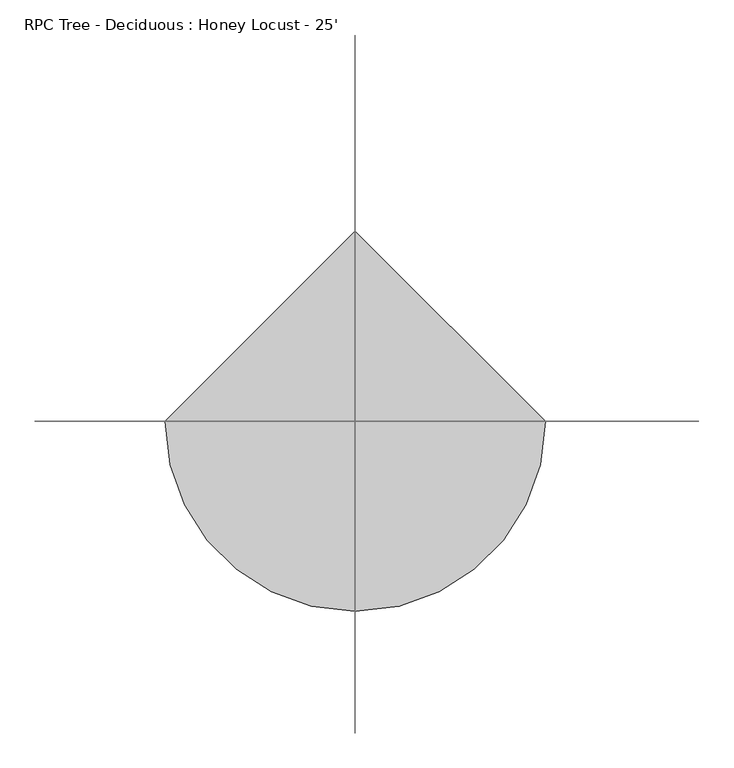
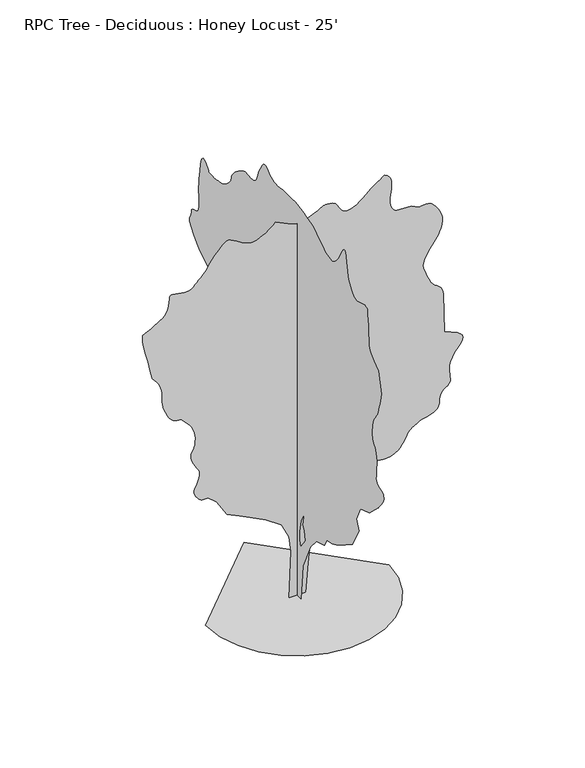
"""IFC4 building model written with IfcOpenShell, lengths in millimetres: geographic element geometry, RPC Tree - Deciduous : Honey Locust - 25'."""

from ifc_helpers import new_model, si_unit, origin, place, context, project, spatial, triangles, source, transform, mapped, element, save


def rpc_tree_deciduous_honey_locust_25_cc46a1f1(model_context):
    return source(origin(), model_context, "Body", "Tessellation", [
        triangles([(0.0017564, 138.2462219, 0.0), (0.0017564, -127.0105432, 0.0), (0.0017564, -184.6753374, 668.9082985), (0.0017564, -426.8668951, 1176.3566122), (0.0017564, -611.3926231, 1395.4822632), (0.0017564, -865.1155083, 1476.2135273), (0.0017564, -934.3152088, 1614.6078415), (0.0017564, -1118.8409369, 1660.7391827), (0.0017564, -1168.1321142, 1679.0297813), (0.0017564, -1234.9772346, 1712.4509972), (0.0017564, -1316.4476978, 1758.4833618), (0.0017564, -1409.6173016, 1814.6021748), (0.0017564, -1511.5651485, 1878.2849155), (0.0017564, -1619.3626385, 1947.0122612), (0.0017564, -1730.0862579, 2018.2590752), (0.0017564, -1937.6776566, 2398.8447109), (0.0017564, -1856.9463924, 2583.3806854), (0.0017564, -1983.8091431, 2848.632518), (0.0017564, -2272.1318058, 2952.4168808), (0.0017564, -2537.389016, 3206.1371498), (0.0017564, -2543.9089668, 3214.0110878), (0.0017564, -2561.3334846, 3235.1946785), (0.0017564, -2586.4031754, 3266.0558762), (0.0017564, -2615.9435234, 3302.9873428), (0.0017564, -2646.6774033, 3342.3317436), (0.0017564, -2675.3794304, 3380.4573235), (0.0017564, -2698.8489281, 3413.7311646), (0.0017564, -2714.4444878, 3444.5414932), (0.0017564, -2721.9882133, 3476.5453537), (0.0017564, -2721.8358971, 3508.1684235), (0.0017564, -2714.4444878, 3537.73377), (0.0017564, -2700.1950668, 3563.6926506), (0.0017564, -2679.4940048, 3584.4190018), (0.0017564, -2652.7226738, 3598.2620522), (0.0017564, -2621.3536583, 3608.345739), (0.0017564, -2588.1556847, 3619.6488281), (0.0017564, -2555.5675575, 3633.3648514), (0.0017564, -2526.024884, 3650.7129204), (0.0017564, -2501.9153091, 3672.9124374), (0.0017564, -2485.67444, 3701.157225), (0.0017564, -2479.7233498, 3736.6663948), (0.0017564, -2481.5749809, 3780.2273987), (0.0017564, -2486.0453476, 3831.0780739), (0.0017564, -2491.5266991, 3887.9740196), (0.0017564, -2496.4008202, 3949.6961243), (0.0017564, -2499.0579254, 4015.0755638), (0.0017564, -2497.8818344, 4082.8426483), (0.0017564, -2491.2575294, 4151.8544243), (0.0017564, -2477.5720276, 4213.7541344), (0.0017564, -2458.0368828, 4262.9284584), (0.0017564, -2435.2733013, 4302.24757), (0.0017564, -2411.9053963, 4334.4801956), (0.0017564, -2390.5542286, 4362.4965088), (0.0017564, -2373.8434753, 4389.0902344), (0.0017564, -2364.3947788, 4417.1062569), (0.0017564, -2359.5864967, 4450.1263344), (0.0017564, -2355.5860142, 4489.1913918), (0.0017564, -2353.1983692, 4533.3113731), (0.0017564, -2353.2315067, 4581.4694801), (0.0017564, -2356.4927902, 4632.6250786), (0.0017564, -2363.7901646, 4685.8128204), (0.0017564, -2375.9288132, 4740.016198), (0.0017564, -2392.0679443, 4787.9461212), (0.0017564, -2410.4271435, 4825.3601166), (0.0017564, -2430.3991802, 4855.916391), (0.0017564, -2451.3794403, 4883.2722794), (0.0017564, -2472.7636002, 4911.0089584), (0.0017564, -2493.9471909, 4942.7843445), (0.0017564, -2514.3232727, 4982.2051941), (0.0017564, -2534.0944496, 5031.4045166), (0.0017564, -2553.8659172, 5089.0626251), (0.0017564, -2573.6269203, 5153.8075104), (0.0017564, -2593.4135033, 5224.1654251), (0.0017564, -2613.1747971, 5298.7905212), (0.0017564, -2632.9360909, 5376.2096329), (0.0017564, -2652.7226738, 5455.0763306), (0.0017564, -2548.9127312, 5835.6443802), (0.0017564, -2410.52612, 5939.4537415), (0.0017564, -2376.165136, 5966.8602081), (0.0017564, -2343.2136589, 5995.5625259), (0.0017564, -2313.0867188, 6026.9059616), (0.0017564, -2287.1965839, 6062.1863663), (0.0017564, -2266.9553776, 6102.6995911), (0.0017564, -2253.772752, 6149.7659042), (0.0017564, -2249.0662079, 6204.705574), (0.0017564, -2247.7225399, 6269.3992996), (0.0017564, -2243.9556187, 6343.7709229), (0.0017564, -2238.1721054, 6426.2187973), (0.0017564, -2230.7756092, 6515.1186035), (0.0017564, -2222.1675591, 6608.8704391), (0.0017564, -2212.7518547, 6705.8220795), (0.0017564, -2202.9347214, 6804.4247818), (0.0017564, -2185.5179066, 6814.1270966), (0.0017564, -2167.3950302, 6822.8393555), (0.0017564, -2147.8598854, 6829.5453415), (0.0017564, -2126.2064106, 6833.2026764), (0.0017564, -2101.7285442, 6832.8218857), (0.0017564, -2073.7199341, 6827.4117508), (0.0017564, -2041.4746639, 6815.9560547), (0.0017564, -2006.8748863, 6801.3255524), (0.0017564, -1972.2775795, 6787.914743), (0.0017564, -1937.6776566, 6776.9165771), (0.0017564, -1903.077879, 6769.5501663), (0.0017564, -1868.4805721, 6767.0357849), (0.0017564, -1833.8806492, 6770.5663834), (0.0017564, -1799.2833424, 6781.3616547), (0.0017564, -1765.6919334, 6801.5546082), (0.0017564, -1733.9191635, 6831.4504578), (0.0017564, -1703.6576385, 6869.42314), (0.0017564, -1674.6050514, 6913.8221741), (0.0017564, -1646.4618565, 6963.0982361), (0.0017564, -1618.9257465, 7015.5746841), (0.0017564, -1591.689473, 7069.6766144), (0.0017564, -1522.4922432, 7484.8646439), (0.0017564, -1510.0182953, 7494.262326), (0.0017564, -1496.8382858, 7500.8665741), (0.0017564, -1482.2460079, 7501.8060516), (0.0017564, -1465.5354, 7494.262326), (0.0017564, -1446.0002552, 7475.4413818), (0.0017564, -1422.9345119, 7442.4974625), (0.0017564, -1395.6321087, 7392.5865555), (0.0017564, -1366.480545, 7335.9952423), (0.0017564, -1337.5296959, 7284.4588531), (0.0017564, -1307.5703327, 7237.3669601), (0.0017564, -1275.393663, 7194.085881), (0.0017564, -1239.7855167, 7154.0296051), (0.0017564, -1199.5366653, 7116.6156097), (0.0017564, -1153.4407871, 7081.2078873), (0.0017564, -1100.9873028, 7057.7133911), (0.0017564, -1043.0880753, 7054.1827927), (0.0017564, -980.6472645, 7067.2889694), (0.0017564, -914.5768787, 7093.7047989), (0.0017564, -845.7836214, 7130.1287384), (0.0017564, -775.1741959, 7173.2069229), (0.0017564, -703.6555235, 7219.6128113), (0.0017564, -659.2741482, 7251.5405136), (0.0017564, -615.4946983, 7282.3758408), (0.0017564, -572.9269114, 7311.0014191), (0.0017564, -532.1751838, 7336.2748764), (0.0017564, -493.8440932, 7357.1282547), (0.0017564, -458.5406522, 7372.4186005), (0.0017564, -426.8668951, 7381.0547012), (0.0017564, -379.7931333, 7391.6464966), (0.0017564, -304.4771091, 7410.7220764), (0.0017564, -210.8004869, 7434.013678), (0.0017564, -108.6519436, 7457.3308594), (0.0017564, -7.915369, 7476.3808594), (0.0017564, 81.5235032, 7486.9726547), (0.0017564, 149.779584, 7484.8646439), (0.0017564, 204.0816928, 7478.1336594), (0.0017564, 257.9799291, 7476.2541229), (0.0017564, 311.0709472, 7476.9907059), (0.0017564, 362.9529548, 7478.1336594), (0.0017564, 413.2194723, 7477.4732346), (0.0017564, 461.4692888, 7472.7485229), (0.0017564, 507.2984682, 7461.8015167), (0.0017564, 555.4821914, 7451.6666702), (0.0017564, 608.9110522, 7450.0156082), (0.0017564, 664.3541433, 7455.4513229), (0.0017564, 718.5906584, 7466.5000671), (0.0017564, 768.3873281, 7481.7909943), (0.0017564, 810.5182594, 7499.9265152), (0.0017564, 841.7526175, 7519.4590439), (0.0017564, 869.6950979, 7543.2081757), (0.0017564, 902.8827524, 7570.9704346), (0.0017564, 939.4967966, 7596.9293152), (0.0017564, 977.728838, 7615.2171524), (0.0017564, 1015.7551506, 7619.9924423), (0.0017564, 1051.7671967, 7605.3875198), (0.0017564, 1083.943939, 7565.5858795), (0.0017564, 1111.584185, 7516.9952408), (0.0017564, 1135.5896965, 7477.701709), (0.0017564, 1156.5725727, 7444.2496811), (0.0017564, 1175.132341, 7413.2114594), (0.0017564, 1191.8760138, 7381.1564392), (0.0017564, 1207.410676, 7344.6819214), (0.0017564, 1222.3407967, 7300.3334656), (0.0017564, 1236.6967518, 7254.9693741), (0.0017564, 1251.0554684, 7217.07285), (0.0017564, 1266.8236919, 7185.6526749), (0.0017564, 1285.4164524, 7159.6432159), (0.0017564, 1308.248489, 7138.103833), (0.0017564, 1336.7269833, 7119.9683121), (0.0017564, 1372.2666744, 7104.2710144), (0.0017564, 1413.6914715, 7095.1529663), (0.0017564, 1457.9408054, 7094.9239105), (0.0017564, 1503.6022625, 7099.7247803), (0.0017564, 1549.2612488, 7105.7447617), (0.0017564, 1593.5105827, 7109.1480423), (0.0017564, 1634.9353798, 7106.0999725), (0.0017564, 1672.1235168, 7092.7397415), (0.0017564, 1714.3205051, 7068.3051865), (0.0017564, 1768.2192501, 7035.5897415), (0.0017564, 1828.5747231, 6996.1944717), (0.0017564, 1890.1391338, 6951.7954376), (0.0017564, 1947.6700699, 6903.9419632), (0.0017564, 1995.9198864, 6854.2845291), (0.0017564, 2029.6434093, 6804.4247818), (0.0017564, 2047.5985634, 6762.5657089), (0.0017564, 2056.0720287, 6732.1873306), (0.0017564, 2061.1140175, 6707.879512), (0.0017564, 2068.7821541, 6684.1809586), (0.0017564, 2085.1219997, 6655.6315384), (0.0017564, 2116.1913242, 6616.7949554), (0.0017564, 2168.0377235, 6562.2360764), (0.0017564, 2230.1762272, 6507.9306702), (0.0017564, 2288.0754547, 6470.9736237), (0.0017564, 2341.7380222, 6447.5297058), (0.0017564, 2391.1637844, 6433.7881027), (0.0017564, 2436.3553574, 6425.8885849), (0.0017564, 2477.3077995, 6419.9959213), (0.0017564, 2514.0259071, 6412.2998795), (0.0017564, 2553.510125, 6405.0352066), (0.0017564, 2599.6366699, 6402.2161926), (0.0017564, 2647.7694878, 6402.6225632), (0.0017564, 2693.3117661, 6405.0352066), (0.0017564, 2731.5640823, 6408.2611725), (0.0017564, 2757.9293335, 6411.0807678), (0.0017564, 2767.7589661, 6412.2998795), (0.0017564, 2779.3922676, 6430.4609802), (0.0017564, 2809.9738312, 6472.8281616), (0.0017564, 2853.0775955, 6521.2403229), (0.0017564, 2902.2519196, 6557.5625244), (0.0017564, 2950.9945839, 6563.6075043), (0.0017564, 2992.9045258, 6521.2403229), (0.0017564, 3021.4792351, 6412.2998795), (0.0017564, 3039.1830963, 6281.2613663), (0.0017564, 3053.0770157, 6180.2965988), (0.0017564, 3063.5417839, 6102.7251709), (0.0017564, 3070.9584824, 6041.8916748), (0.0017564, 3075.7846413, 5991.1680267), (0.0017564, 3078.3751808, 5943.8482407), (0.0017564, 3079.1373436, 5893.3274872), (0.0017564, 3077.918232, 5838.9459229), (0.0017564, 3075.0986366, 5784.5899384), (0.0017564, 3071.8729614, 5730.2089554), (0.0017564, 3069.4600273, 5675.8273911), (0.0017564, 3069.0536568, 5621.4714066), (0.0017564, 3071.8729614, 5567.0904236), (0.0017564, 3079.1373436, 5512.7344391), (0.0017564, 3099.1779808, 5469.782991), (0.0017564, 3134.966494, 5444.6112717), (0.0017564, 3179.5942932, 5429.5238205), (0.0017564, 3226.2792343, 5416.8495941), (0.0017564, 3268.113018, 5398.9169678), (0.0017564, 3298.2376328, 5368.0816406), (0.0017564, 3309.7944855, 5316.6719879), (0.0017564, 3318.6843498, 5264.1193817), (0.0017564, 3338.4456436, 5228.1023941), (0.0017564, 3358.8164932, 5198.3588608), (0.0017564, 3369.5097359, 5164.551622), (0.0017564, 3360.2387901, 5116.4440933), (0.0017564, 3320.6912041, 5043.7235321), (0.0017564, 3240.6051041, 4936.0789398), (0.0017564, 3137.9128258, 4824.090136), (0.0017564, 3039.0560692, 4740.5243065), (0.0017564, 2946.4477684, 4678.5737274), (0.0017564, 2862.5264374, 4631.3298088), (0.0017564, 2789.7047195, 4591.9598282), (0.0017564, 2730.395549, 4553.5804848), (0.0017564, 2687.0124413, 4509.3590561), (0.0017564, 2658.1580978, 4464.7821259), (0.0017564, 2638.3970947, 4426.6568367), (0.0017564, 2624.0715157, 4390.1317406), (0.0017564, 2611.574604, 4350.4059677), (0.0017564, 2597.249025, 4302.5777824), (0.0017564, 2577.462442, 4241.8466057), (0.0017564, 2548.6333878, 4163.3859879), (0.0017564, 2517.7242279, 4078.1182274), (0.0017564, 2493.4823936, 3999.5052933), (0.0017564, 2474.7855698, 3926.4298119), (0.0017564, 2460.5312073, 3857.7988266), (0.0017564, 2449.6039673, 3792.521125), (0.0017564, 2440.8943245, 3729.4275925), (0.0017564, 2433.294643, 3667.4770134), (0.0017564, 2455.3521629, 3642.6102173), (0.0017564, 2476.2994308, 3616.9562599), (0.0017564, 2495.0267761, 3589.7021095), (0.0017564, 2510.4267082, 3560.0097359), (0.0017564, 2521.3894112, 3527.0913963), (0.0017564, 2526.8021622, 3490.1343498), (0.0017564, 2525.5600868, 3448.3514351), (0.0017564, 2526.3652702, 3406.9748909), (0.0017564, 2533.4264671, 3370.2718987), (0.0017564, 2538.8723557, 3335.7786552), (0.0017564, 2534.8385902, 3301.0569374), (0.0017564, 2513.4544304, 3263.7443893), (0.0017564, 2466.850589, 3221.3772079), (0.0017564, 2387.1633018, 3171.5424591), (0.0017564, 2299.4063038, 3131.0039452), (0.0017564, 2230.2092194, 3111.2173622), (0.0017564, 2174.1235439, 3101.9464165), (0.0017564, 2125.7061504, 3092.878656), (0.0017564, 2079.5060635, 3073.7016289), (0.0017564, 2030.0803013, 3034.1540428), (0.0017564, 1971.9778885, 2963.9484444), (0.0017564, 1918.922406, 2886.046804), (0.0017564, 1885.02869, 2826.5091591), (0.0017564, 1865.4579369, 2779.671611), (0.0017564, 1855.3716339, 2739.8952599), (0.0017564, 1849.9258907, 2701.5159164), (0.0017564, 1844.2769623, 2658.9202606), (0.0017564, 1833.5835743, 2606.4438126), (0.0017564, 1823.3625412, 2556.2026932), (0.0017564, 1818.1834969, 2520.8993248), (0.0017564, 1811.7953693, 2495.6822594), (0.0017564, 1797.9422905, 2475.7102226), (0.0017564, 1770.3705723, 2456.1393242), (0.0017564, 1722.8269627, 2432.1339581), (0.0017564, 1649.0577736, 2398.8447109), (0.0017564, 1567.2851486, 2366.9372108), (0.0017564, 1497.6180347, 2346.9297112), (0.0017564, 1436.6226299, 2333.7851646), (0.0017564, 1380.8747246, 2322.4516994), (0.0017564, 1326.9429874, 2307.8950298), (0.0017564, 1271.3957966, 2285.0629932), (0.0017564, 1210.806617, 2248.9188332), (0.0017564, 1144.870816, 2202.0812851), (0.0017564, 1075.9099091, 2151.0044609), (0.0017564, 1004.4242289, 2096.4021252), (0.0017564, 930.9242821, 2038.9727818), (0.0017564, 855.9105469, 1979.4251083), (0.0017564, 779.8858995, 1918.4651665), (0.0017564, 703.3583033, 1856.7991631), (0.0017564, 276.64129, 1533.8765774), (0.0017564, 149.779584, 1314.7509991), (0.0017564, 115.1805058, 1141.7593054), (0.0017564, 103.6476433, 876.5023132), (0.0020752, -103.9448272, 980.2967772), (0.0020752, -80.8791112, 1107.1595278), (0.0020752, -80.8791112, 1268.6195126), (0.0020752, -127.0105432, 1499.2792706), (0.0020752, -230.8067694, 1706.8706692), (0.0020752, -184.6753374, 1453.147784), (0.0020752, -230.8067694, 1372.4165199), (0.0020752, -265.4043305, 1199.4223555), (154.7882082, 0.0004434, 0.0162828), (-145.0671264, 0.0004434, 0.0162828), (-110.4685569, 0.0003925, 876.5175739), (-145.0671264, 0.000378, 1164.8403093), (-283.4611681, 0.0003635, 1441.6288651), (-560.2523217, 0.0003489, 1637.6887001), (-963.9036644, 0.0003344, 1845.2827148), (-1263.7605068, 0.0003271, 1983.677029), (-1459.8203419, 0.0003126, 2295.065435), (-1609.7462196, 0.000298, 2421.9281857), (-1636.8810459, 0.0003053, 2419.6396626), (-1663.7135651, 0.0003053, 2418.4637169), (-1689.9389992, 0.0003053, 2419.5050777), (-1715.2578026, 0.000298, 2423.8764679), (-1739.3649067, 0.000298, 2432.6877033), (-1761.9606205, 0.000298, 2447.0436584), (-1782.7404568, 0.000298, 2468.0595268), (-1802.9155334, 0.000298, 2493.4774521), (-1822.6843849, 0.000298, 2520.3098259), (-1840.2357845, 0.0002908, 2548.5572296), (-1853.7537094, 0.0002908, 2578.199025), (-1861.4193752, 0.0002908, 2609.2886971), (-1861.4193752, 0.0002908, 2641.7497971), (-1851.9375412, 0.0002835, 2675.6587738), (-1833.5784874, 0.0002835, 2714.1904335), (-1810.985099, 0.0002835, 2759.3769196), (-1788.3893852, 0.0002762, 2809.4148537), (-1770.0301861, 0.0002762, 2862.4755684), (-1760.1445976, 0.000269, 2916.7298149), (-1762.9689892, 0.000269, 2970.4000854), (-1782.7404568, 0.000269, 3021.631842), (-1812.8012672, 0.0002617, 3069.7646599), (-1842.4557072, 0.0002617, 3115.6624397), (-1869.8928406, 0.0002544, 3159.9347374), (-1893.2963539, 0.0002544, 3203.2161072), (-1910.8477535, 0.0002544, 3246.0658173), (-1920.7308712, 0.0002471, 3289.1442924), (-1921.134771, 0.0002471, 3333.0355087), (-1913.6366821, 0.0002471, 3370.6526894), (-1902.1049732, 0.0002399, 3398.1864738), (-1888.1503017, 0.0002399, 3421.0972847), (-1873.3903015, 0.0002399, 3444.7952568), (-1859.43563, 0.0002399, 3474.7419754), (-1847.9014503, 0.0002399, 3516.397863), (-1840.4059776, 0.0002326, 3575.2242142), (-1839.1614315, 0.0002253, 3640.3751793), (-1844.5740372, 0.0002253, 3698.2870514), (-1855.534124, 0.0002253, 3750.1283638), (-1870.9342014, 0.0002181, 3797.143808), (-1889.6641628, 0.0002181, 3840.5016266), (-1910.6114307, 0.0002181, 3881.4718002), (-1932.6688053, 0.0002108, 3921.1972824), (-2094.1288628, 0.0002035, 4094.1966064), (-2131.1822697, 0.0002035, 4094.6791351), (-2168.1342293, 0.0002035, 4097.9556793), (-2204.8854744, 0.0002035, 4106.8964127), (-2241.3344124, 0.0002035, 4124.3209305), (-2277.3769798, 0.0001963, 4153.0482468), (-2312.9191418, 0.0001963, 4195.8726677), (-2347.8542187, 0.000189, 4255.6640762), (-2378.9895275, 0.000189, 4321.6024933), (-2403.4675392, 0.0001817, 4382.0799065), (-2421.6893921, 0.0001817, 4438.7470871), (-2434.0643635, 0.0001817, 4493.1792297), (-2440.9908302, 0.0001745, 4547.0018166), (-2442.8729828, 0.0001745, 4601.8403297), (-2440.1170464, 0.0001672, 4659.3205421), (-2439.9138611, 0.0001672, 4717.8166809), (-2448.3874718, 0.0001599, 4774.3062561), (-2464.3234177, 0.0001599, 4828.1797119), (-2486.5177025, 0.0001527, 4878.801622), (-2513.751796, 0.0001527, 4925.6138809), (-2544.8234459, 0.0001527, 4967.9810623), (-2578.5039482, 0.0001454, 5005.2933197), (-2606.1136002, 0.0001454, 5036.2053864), (-2622.8268242, 0.0001454, 5064.6786484), (-2633.2915924, 0.0001454, 5098.2068344), (-2642.1308784, 0.0001381, 5144.2313507), (-2653.9926544, 0.0001381, 5210.2459259), (-2673.5251831, 0.0001308, 5303.6669678), (-2705.3767273, 0.0001236, 5432.0132034), (-2739.5397583, 0.0001163, 5564.8295151), (-2764.0251823, 0.000109, 5669.807991), (-2780.4334831, 0.0001018, 5751.5704422), (-2790.3651443, 0.0001018, 5814.7910019), (-2795.4959358, 9.45e-05, 5864.0920624), (-2797.3754723, 9.45e-05, 5904.0971786), (-2797.6295265, 9.45e-05, 5939.4537415), (-2780.0526924, 9.45e-05, 5947.0736252), (-2760.7486382, 9.45e-05, 5955.7608856), (-2738.0157234, 8.72e-05, 5966.7078918), (-2710.1520172, 8.72e-05, 5980.9576035), (-2675.4047195, 8.72e-05, 5999.6518112), (-2632.0977699, 8.72e-05, 6023.8834717), (-2578.5039482, 8.72e-05, 6054.794957), (-2522.6948547, 8e-05, 6086.4941849), (-2473.739122, 8e-05, 6114.9674469), (-2431.4405411, 8e-05, 6144.0761353), (-2395.5985428, 8e-05, 6177.5787415), (-2366.0102325, 7.27e-05, 6219.387236), (-2342.4746052, 7.27e-05, 6273.2856903), (-2324.7886208, 6.54e-05, 6343.110498), (-2314.1282249, 6.54e-05, 6412.6556717), (-2308.7154739, 5.82e-05, 6464.4205353), (-2303.9071918, 5.82e-05, 6500.4631027), (-2295.0629642, 5.82e-05, 6522.7896469), (-2277.5471729, 5.82e-05, 6533.4320206), (-2246.7141712, 5.82e-05, 6534.3720795), (-2197.9258701, 5.82e-05, 6527.641095), (-2140.092627, 5.82e-05, 6517.4300903), (-2085.4878204, 5.82e-05, 6508.0068283), (-2034.5150597, 5.82e-05, 6501.6060562), (-1987.575919, 5.82e-05, 6500.4631027), (-1945.0767689, 5.82e-05, 6506.7877167), (-1907.4187477, 5.82e-05, 6522.7896469), (-1875.0032845, 5.82e-05, 6550.7042221), (-1844.541045, 5.09e-05, 6583.0894547), (-1812.0595974, 5.09e-05, 6613.4422531), (-1776.9567982, 5.09e-05, 6645.4205338), (-1738.6257076, 5.09e-05, 6682.6572144), (-1696.4617115, 4.36e-05, 6728.7578888), (-1649.8604862, 4.36e-05, 6787.3560562), (-1598.2146561, 3.63e-05, 6862.1078888), (-1546.1980637, 2.91e-05, 6938.7142593), (-1498.4181313, 2.91e-05, 7002.036557), (-1454.1714134, 2.91e-05, 7054.2589508), (-1412.7466164, 2.18e-05, 7097.5911896), (-1373.4401493, 2.18e-05, 7134.268602), (-1335.5459507, 2.18e-05, 7166.5265167), (-1298.3578136, 1.45e-05, 7196.5496841), (-1288.0707962, 1.45e-05, 7208.5129074), (-1275.3606709, 1.45e-05, 7218.1646439), (-1257.8092712, 1.45e-05, 7223.193988), (-1232.9934895, 1.45e-05, 7221.2382935), (-1198.4952318, 1.45e-05, 7210.0116531), (-1151.8939339, 1.45e-05, 7187.1770004), (-1090.7663424, 2.18e-05, 7150.4228485), (-1026.7456861, 2.18e-05, 7109.5544128), (-971.2010387, 2.18e-05, 7076.382019), (-921.3027763, 2.91e-05, 7051.4649353), (-874.2290508, 2.91e-05, 7035.4374252), (-827.1577961, 2.91e-05, 7028.858757), (-777.2595337, 2.91e-05, 7032.3893555), (-721.7123428, 2.91e-05, 7046.6134872), (-664.755427, 2.18e-05, 7068.7365555), (-612.0327003, 2.18e-05, 7095.1018066), (-562.8405722, 2.18e-05, 7124.9976563), (-516.4729082, 2.18e-05, 7157.7131012), (-472.226154, 1.45e-05, 7192.5615555), (-429.3891249, 1.45e-05, 7228.8075989), (-387.2581573, 1.45e-05, 7265.7390656), (-168.1328515, 2.18e-05, 7161.9547028), (-133.3996518, 2.18e-05, 7144.8603973), (-97.8597517, 2.18e-05, 7129.1125214), (-60.7056832, 2.18e-05, 7115.9551849), (-21.1306711, 2.18e-05, 7106.7348175), (21.6722237, 2.18e-05, 7102.77285), (68.5100806, 2.18e-05, 7105.3633896), (120.1896296, 2.18e-05, 7115.8284485), (179.9390167, 2.18e-05, 7135.6656097), (246.5473965, 2.18e-05, 7162.9709198), (314.1646537, 1.45e-05, 7193.9079849), (376.9406911, 1.45e-05, 7224.6165756), (429.0233405, 1.45e-05, 7251.3120392), (464.5629953, 1.45e-05, 7270.1585632), (477.7100126, 1.45e-05, 7277.2703384), (487.5271096, 1.45e-05, 7279.4550888), (513.8897447, 1.45e-05, 7283.4682159), (552.1522711, 1.45e-05, 7285.4494904), (597.6791797, 1.45e-05, 7281.5886795), (645.8273672, 1.45e-05, 7268.0249725), (691.9587811, 1.45e-05, 7240.9737167), (731.4328978, 1.45e-05, 7196.5496841), (761.0238968, 2.18e-05, 7148.2642593), (783.1472557, 2.18e-05, 7111.0787384), (801.640967, 2.18e-05, 7083.3670578), (820.3353928, 2.18e-05, 7063.5298965), (843.065764, 2.91e-05, 7049.9406097), (873.6625883, 2.91e-05, 7040.9998764), (915.9611692, 2.91e-05, 7035.081633), (967.9092339, 2.91e-05, 7039.3999741), (1023.6901314, 2.18e-05, 7059.6435059), (1081.4903097, 2.18e-05, 7091.9775787), (1139.4911299, 2.18e-05, 7132.5925415), (1195.8764963, 1.45e-05, 7177.6520004), (1248.8354004, 1.45e-05, 7223.3207245), (1296.5467323, 1.45e-05, 7265.7390656), (1340.3591743, 7.3e-06, 7303.2803787), (1382.9600624, 7.3e-06, 7337.1637756), (1424.5524364, 7.3e-06, 7368.0246826), (1465.3373016, 7.3e-06, 7396.4723648), (1505.5174072, 0.0, 7423.1172501), (1545.2937584, 0.0, 7448.5168625), (1584.8695404, 0.0, 7473.3327896), (1611.8696365, 0.0, 7460.5568253), (1637.7599167, 0.0, 7445.2658981), (1661.4301289, 0.0, 7424.9206284), (1681.7729279, 7.3e-06, 7397.0060532), (1697.6758816, 7.3e-06, 7359.0327896), (1708.0339703, 7.3e-06, 7308.4108795), (1711.732291, 1.45e-05, 7242.6759384), (1708.6384392, 2.18e-05, 7173.2069229), (1701.1073582, 2.18e-05, 7112.0182159), (1691.7602543, 2.18e-05, 7057.4843353), (1683.2181885, 2.91e-05, 7007.9797989), (1678.1077446, 2.91e-05, 6961.9297028), (1679.0501289, 3.63e-05, 6917.6829849), (1688.6665478, 3.63e-05, 6873.639743), (1703.4950031, 3.63e-05, 6833.8631012), (1718.3209877, 4.36e-05, 6802.5452454), (1733.1494431, 4.36e-05, 6778.3135849), (1747.9780437, 4.36e-05, 6759.7205338), (1762.8064991, 4.36e-05, 6745.3440857), (1777.6324837, 4.36e-05, 6733.8128128), (1792.460939, 4.36e-05, 6723.7035461), (2069.2520382, 4.36e-05, 6712.1716919), (2207.6463524, 5.09e-05, 6642.9823105), (2217.499094, 5.09e-05, 6645.8524841), (2244.0954357, 5.09e-05, 6651.9742035), (2282.9953869, 5.09e-05, 6657.485495), (2329.7669506, 5.09e-05, 6658.5778702), (2379.9675201, 5.09e-05, 6651.3899368), (2429.1595757, 5.09e-05, 6632.0858826), (2472.9034172, 5.09e-05, 6596.8304764), (2512.6797684, 5.82e-05, 6549.0025818), (2551.0463219, 5.82e-05, 6495.1035461), (2585.1840637, 6.54e-05, 6436.1501678), (2612.2350288, 6.54e-05, 6373.1836624), (2629.4307816, 7.27e-05, 6307.1690872), (2633.9011482, 7.27e-05, 6239.1482391), (2622.8268242, 8e-05, 6170.111174), (2602.049604, 8e-05, 6105.620343), (2579.4690056, 8.72e-05, 6049.6132965), (2555.3390831, 8.72e-05, 6000.6680283), (2530.0304535, 8.72e-05, 5957.360788), (2503.8024033, 9.45e-05, 5918.2701508), (2476.9726456, 9.45e-05, 5882.0246887), (2449.837674, 9.45e-05, 5847.2012329), (2408.2121624, 0.0001018, 5785.5299973), (2368.9058407, 0.0001018, 5724.5703461), (2334.2399334, 0.000109, 5665.0327011), (2306.5336304, 0.000109, 5607.603067), (2288.1084469, 0.0001163, 5552.9930283), (2281.2834274, 0.0001163, 5501.9141693), (2288.3777618, 0.0001236, 5455.0763306), (2303.2722015, 0.0001236, 5411.8202499), (2318.5706863, 0.0001236, 5370.1390732), (2334.6768253, 0.0001308, 5328.8892654), (2351.9919022, 0.0001308, 5286.8267166), (2370.922578, 0.0001308, 5242.7578949), (2391.869846, 0.0001381, 5195.4375275), (2415.2378963, 0.0001381, 5143.6982437), (2445.5678764, 0.0001454, 5097.4190918), (2484.1684273, 0.0001454, 5063.0531662), (2526.5989769, 0.0001454, 5034.1479538), (2568.4199707, 0.0001454, 5004.2265244), (2605.2247009, 0.0001527, 4966.8381088), (2632.5041405, 0.0001527, 4915.5301941), (2645.8899513, 0.0001599, 4843.8258499), (2668.9530785, 0.0002035, 4105.72817), (2899.6102203, 0.0002108, 4001.9438072), (2935.957711, 0.0002108, 3979.3123398), (2967.9871513, 0.0002108, 3954.3696762), (2991.3043327, 0.0002108, 3924.7787498), (3001.6420738, 0.0002108, 3888.2280739), (2994.6061661, 0.0002181, 3842.381163), (2965.9041389, 0.0002181, 3784.9518196), (2911.1417839, 0.0002253, 3713.6032677), (2850.7916885, 0.0002326, 3637.2509514), (2806.7987343, 0.0002326, 3565.9279793), (2777.1063606, 0.0002399, 3499.049794), (2759.707132, 0.0002399, 3436.0068398), (2752.6206459, 0.0002471, 3376.1901421), (2753.7891792, 0.0002471, 3319.0145622), (2761.2311668, 0.0002544, 3263.8205475), (2769.4861862, 0.0002544, 3214.1381149), (2773.7280785, 0.0002544, 3172.7107018), (2772.7374413, 0.0002617, 3137.9384056), (2765.2698738, 0.0002617, 3108.2201614), (2750.1315536, 0.0002617, 3081.9313591), (2726.1283676, 0.0002617, 3057.4456444), (2692.0162056, 0.0002617, 3033.1634056), (2656.5834846, 0.000269, 3007.7126335), (2628.8212257, 0.000269, 2980.6616684), (2607.8916893, 0.000269, 2951.756456), (2593.0327126, 0.000269, 2920.8699692), (2583.4315544, 0.0002762, 2887.7484444), (2578.249894, 0.0002762, 2852.2139854), (2576.7002792, 0.0002762, 2814.0378273), (2574.4905304, 0.0002835, 2776.5473831), (2567.4293335, 0.0002835, 2742.8924606), (2554.9071327, 0.0002835, 2712.6663986), (2536.3501259, 0.0002835, 2685.4631172), (2511.1330605, 0.0002908, 2660.9012444), (2478.6539383, 0.0002908, 2638.5238312), (2438.3036396, 0.0002908, 2617.9753761), (2396.3758209, 0.0002908, 2601.9734459), (2358.4816223, 0.0002908, 2591.6357048), (2323.0080608, 0.0002908, 2584.0916885), (2288.3421535, 0.0002908, 2576.5735428), (2252.8710629, 0.0002908, 2566.2102219), (2214.9768642, 0.0002908, 2550.2082916), (2173.0465748, 0.000298, 2525.7225769), (2134.3801849, 0.000298, 2501.648465), (2105.1956291, 0.000298, 2485.6439186), (2082.2644707, 0.000298, 2473.0685234), (2062.3585636, 0.000298, 2459.2838997), (2042.2519421, 0.000298, 2439.6473076), (2018.7163147, 0.0003053, 2409.5203674), (1988.5207741, 0.0003053, 2364.2626648), (1957.3856106, 0.0003053, 2310.7346821), (1930.083062, 0.0003126, 2259.4242966), (1901.9730045, 0.0003126, 2211.1414879), (1868.4170586, 0.0003198, 2166.6889687), (1824.7748096, 0.0003198, 2126.8796253), (1766.4030819, 0.0003198, 2092.5158798), (1688.6665478, 0.0003198, 2064.4058224), (1611.2981598, 0.0003271, 2049.7144226), (1552.6928707, 0.0003271, 2049.9481293), (1506.1906219, 0.0003198, 2057.4462181), (1465.1365871, 0.0003198, 2064.5404072), (1422.8709984, 0.0003198, 2063.5676468), (1372.7390293, 0.0003271, 2046.8544228), (1308.0784412, 0.0003271, 2006.7427723), (1236.0922829, 0.0003271, 1957.583709), (1168.5411009, 0.0003344, 1917.1011509), (1105.630406, 0.0003344, 1882.6715664), (1047.5635288, 0.0003344, 1851.6708424), (994.5385677, 0.0003344, 1821.4753017), (946.7611788, 0.0003416, 1789.4663544), (904.4270622, 0.0003416, 1753.0174164), (863.5407497, 0.0003416, 1713.1393272), (820.2337275, 0.0003489, 1672.6569145), (774.9100405, 0.0003489, 1631.6714802), (727.9708998, 0.0003489, 1590.2796753), (679.8201324, 0.0003562, 1548.5857086), (630.8642544, 0.0003562, 1506.6908821), (581.50702, 0.0003562, 1464.6946083), (339.3157348, 0.000378, 1176.3718729), (235.5192361, 0.0003925, 899.5832445), (200.9196402, 0.0004143, 542.0633883), (-1658.5903313, 0.0, 0.0172132), (-1614.7424263, -380.0394845, 0.0172132), (-1489.866037, -729.0453255, 0.0172132), (-1293.9560474, -1037.0174429, 0.0172132), (-1037.0174429, -1293.9560474, 0.0172132), (-729.0453255, -1489.866037, 0.0172132), (-380.0394845, -1614.7424263, 0.0172132), (7.25e-05, -1658.5903313, 0.0172132), (380.0394845, -1614.7424263, 0.0172132), (729.0453255, -1489.866037, 0.0172132), (1037.0174429, -1293.9560474, 0.0172132), (1293.9560474, -1037.0174429, 0.0172132), (1489.866037, -729.0453255, 0.0172132), (1614.7424263, -380.0394845, 0.0172132), (1658.5903313, 0.0001454, 0.0172132), (-0.0002175, 1658.5903313, 0.0172132)], [[328, 1, 329], [327, 328, 329], [327, 329, 330], [329, 1, 2], [329, 2, 3], [329, 3, 4], [336, 329, 4], [327, 330, 331], [326, 327, 331], [326, 331, 332], [325, 326, 332], [335, 336, 4], [335, 4, 5], [325, 332, 333], [334, 335, 5], [333, 334, 5], [333, 5, 6], [333, 6, 7], [324, 325, 333], [91, 92, 93], [223, 224, 225], [222, 223, 225], [222, 225, 226], [221, 222, 226], [220, 221, 226], [220, 226, 227], [219, 220, 227], [219, 227, 228], [15, 16, 17], [91, 93, 94], [91, 94, 95], [91, 95, 96], [91, 96, 97], [91, 97, 98], [91, 98, 99], [91, 99, 100], [90, 91, 100], [90, 100, 101], [90, 101, 102], [89, 90, 102], [89, 102, 103], [88, 89, 103], [88, 103, 104], [218, 219, 228], [14, 15, 17], [218, 228, 229], [217, 218, 229], [216, 217, 229], [216, 229, 230], [215, 216, 230], [215, 230, 231], [214, 215, 231], [214, 231, 232], [214, 232, 233], [214, 233, 234], [213, 214, 234], [213, 234, 235], [113, 114, 115], [113, 115, 116], [113, 116, 117], [113, 117, 118], [113, 118, 119], [113, 119, 120], [113, 120, 121], [113, 121, 122], [113, 122, 123], [113, 123, 124], [113, 124, 125], [113, 125, 126], [113, 126, 127], [112, 113, 127], [112, 127, 128], [111, 112, 128], [110, 111, 128], [213, 235, 236], [87, 88, 104], [87, 104, 105], [212, 213, 236], [110, 128, 129], [109, 110, 129], [212, 236, 237], [211, 212, 237], [210, 211, 237], [86, 87, 105], [210, 237, 238], [209, 210, 238], [85, 86, 105], [76, 77, 78], [75, 76, 78], [13, 14, 17], [209, 238, 239], [85, 105, 106], [208, 209, 239], [74, 75, 78], [108, 109, 129], [74, 78, 79], [73, 74, 79], [84, 85, 106], [73, 79, 80], [72, 73, 80], [71, 72, 80], [208, 239, 240], [70, 71, 80], [69, 70, 80], [68, 69, 80], [67, 68, 80], [66, 67, 80], [65, 66, 80], [65, 80, 81], [64, 65, 81], [12, 13, 17], [245, 246, 247], [244, 245, 247], [243, 244, 247], [243, 247, 248], [64, 81, 82], [63, 64, 82], [242, 243, 248], [323, 324, 333], [167, 168, 169], [167, 169, 170], [166, 167, 170], [166, 170, 171], [165, 166, 171], [164, 165, 171], [164, 171, 172], [163, 164, 172], [163, 172, 173], [163, 173, 174], [162, 163, 174], [162, 174, 175], [162, 175, 176], [162, 176, 177], [161, 162, 177], [161, 177, 178], [161, 178, 179], [160, 161, 179], [160, 179, 180], [159, 160, 180], [159, 180, 181], [158, 159, 181], [11, 12, 17], [250, 251, 252], [249, 250, 252], [249, 252, 253], [248, 249, 253], [242, 248, 253], [242, 253, 254], [242, 254, 255], [241, 242, 255], [241, 255, 256], [241, 256, 257], [241, 257, 258], [241, 258, 259], [240, 241, 259], [208, 240, 259], [208, 259, 260], [208, 260, 261], [207, 208, 261], [206, 207, 261], [206, 261, 262], [206, 262, 263], [205, 206, 263], [205, 263, 264], [204, 205, 264], [204, 264, 265], [204, 265, 266], [204, 266, 267], [204, 267, 268], [204, 268, 269], [203, 204, 269], [10, 11, 17], [9, 10, 17], [8, 9, 17], [7, 8, 17], [333, 7, 17], [323, 333, 17], [322, 323, 17], [322, 17, 18], [321, 322, 18], [320, 321, 18], [319, 320, 18], [318, 319, 18], [317, 318, 18], [316, 317, 18], [315, 316, 18], [203, 269, 270], [314, 315, 18], [18, 19, 20], [314, 18, 20], [314, 20, 21], [314, 21, 22], [314, 22, 23], [314, 23, 24], [314, 24, 25], [314, 25, 26], [314, 26, 27], [314, 27, 28], [314, 28, 29], [314, 29, 30], [314, 30, 31], [314, 31, 32], [314, 32, 33], [314, 33, 34], [314, 34, 35], [314, 35, 36], [314, 36, 37], [314, 37, 38], [314, 38, 39], [314, 39, 40], [314, 40, 41], [314, 41, 42], [314, 42, 43], [314, 43, 44], [314, 44, 45], [314, 45, 46], [314, 46, 47], [314, 47, 48], [314, 48, 49], [314, 49, 50], [314, 50, 51], [314, 51, 52], [314, 52, 53], [314, 53, 54], [314, 54, 55], [314, 55, 56], [314, 56, 57], [314, 57, 58], [314, 58, 59], [314, 59, 60], [314, 60, 61], [314, 61, 62], [313, 314, 62], [312, 313, 62], [311, 312, 62], [310, 311, 62], [309, 310, 62], [308, 309, 62], [307, 308, 62], [306, 307, 62], [305, 306, 62], [304, 305, 62], [303, 304, 62], [302, 303, 62], [301, 302, 62], [300, 301, 62], [299, 300, 62], [298, 299, 62], [297, 298, 62], [296, 297, 62], [295, 296, 62], [294, 295, 62], [294, 62, 63], [294, 63, 82], [294, 82, 83], [294, 83, 84], [294, 84, 106], [294, 106, 107], [294, 107, 108], [294, 108, 129], [294, 129, 130], [294, 130, 131], [294, 131, 132], [294, 132, 133], [294, 133, 134], [294, 134, 135], [294, 135, 136], [294, 136, 137], [294, 137, 138], [294, 138, 139], [294, 139, 140], [294, 140, 141], [294, 141, 142], [294, 142, 143], [294, 143, 144], [294, 144, 145], [294, 145, 146], [294, 146, 147], [294, 147, 148], [294, 148, 149], [294, 149, 150], [294, 150, 151], [294, 151, 152], [294, 152, 153], [294, 153, 154], [294, 154, 155], [294, 155, 156], [294, 156, 157], [294, 157, 158], [294, 158, 181], [294, 181, 182], [294, 182, 183], [294, 183, 184], [294, 184, 185], [293, 294, 185], [293, 185, 186], [293, 186, 187], [292, 293, 187], [292, 187, 188], [292, 188, 189], [292, 189, 190], [292, 190, 191], [292, 191, 192], [292, 192, 193], [292, 193, 194], [292, 194, 195], [292, 195, 196], [292, 196, 197], [292, 197, 198], [292, 198, 199], [292, 199, 200], [292, 200, 201], [292, 201, 202], [292, 202, 203], [292, 203, 270], [292, 270, 271], [292, 271, 272], [292, 272, 273], [292, 273, 274], [292, 274, 275], [291, 292, 275], [290, 291, 275], [289, 290, 275], [289, 275, 276], [289, 276, 277], [289, 277, 278], [289, 278, 279], [289, 279, 280], [289, 280, 281], [289, 281, 282], [289, 282, 283], [288, 289, 283], [288, 283, 284], [287, 288, 284], [286, 287, 284], [285, 286, 284], [337, 338, 339], [677, 337, 339], [676, 677, 339], [676, 339, 340], [675, 676, 340], [423, 424, 425], [486, 487, 488], [675, 340, 341], [674, 675, 341], [529, 530, 531], [485, 486, 488], [484, 485, 488], [423, 425, 426], [529, 531, 532], [673, 674, 341], [673, 341, 342], [672, 673, 342], [671, 672, 342], [670, 671, 342], [669, 670, 342], [668, 669, 342], [667, 668, 342], [529, 532, 533], [528, 529, 533], [528, 533, 534], [528, 534, 535], [528, 535, 536], [527, 528, 536], [527, 536, 537], [526, 527, 537], [526, 537, 538], [525, 526, 538], [525, 538, 539], [524, 525, 539], [524, 539, 540], [523, 524, 540], [523, 540, 541], [522, 523, 541], [522, 541, 542], [521, 522, 542], [521, 542, 543], [520, 521, 543], [519, 520, 543], [519, 543, 544], [519, 544, 545], [518, 519, 545], [518, 545, 546], [517, 518, 546], [517, 546, 547], [422, 423, 426], [422, 426, 427], [441, 442, 443], [441, 443, 444], [440, 441, 444], [440, 444, 445], [439, 440, 445], [439, 445, 446], [438, 439, 446], [438, 446, 447], [438, 447, 448], [437, 438, 448], [437, 448, 449], [666, 667, 342], [421, 422, 427], [421, 427, 428], [421, 428, 429], [420, 421, 429], [420, 429, 430], [419, 420, 430], [419, 430, 431], [418, 419, 431], [418, 431, 432], [418, 432, 433], [417, 418, 433], [417, 433, 434], [416, 417, 434], [483, 484, 488], [436, 437, 449], [343, 344, 345], [666, 342, 343], [666, 343, 345], [665, 666, 345], [664, 665, 345], [663, 664, 345], [662, 663, 345], [661, 662, 345], [660, 661, 345], [659, 660, 345], [659, 345, 346], [517, 547, 548], [483, 488, 489], [416, 434, 435], [415, 416, 435], [482, 483, 489], [482, 489, 490], [436, 449, 450], [658, 659, 346], [414, 415, 435], [600, 601, 602], [599, 600, 602], [599, 602, 603], [598, 599, 603], [597, 598, 603], [597, 603, 604], [596, 597, 604], [596, 604, 605], [596, 605, 606], [596, 606, 607], [596, 607, 608], [516, 517, 548], [516, 548, 549], [413, 414, 435], [412, 413, 435], [411, 412, 435], [410, 411, 435], [409, 410, 435], [408, 409, 435], [407, 408, 435], [407, 435, 436], [407, 436, 450], [407, 450, 451], [406, 407, 451], [405, 406, 451], [405, 451, 452], [404, 405, 452], [404, 452, 453], [404, 453, 454], [404, 454, 455], [404, 455, 456], [551, 552, 553], [482, 490, 491], [481, 482, 491], [404, 456, 457], [467, 468, 469], [467, 469, 470], [466, 467, 470], [466, 470, 471], [466, 471, 472], [465, 466, 472], [465, 472, 473], [464, 465, 473], [463, 464, 473], [463, 473, 474], [462, 463, 474], [461, 462, 474], [461, 474, 475], [460, 461, 475], [459, 460, 475], [459, 475, 476], [458, 459, 476], [458, 476, 477], [457, 458, 477], [404, 457, 477], [404, 477, 478], [404, 478, 479], [404, 479, 480], [403, 404, 480], [403, 480, 481], [403, 481, 491], [403, 491, 492], [403, 492, 493], [402, 403, 493], [401, 402, 493], [400, 401, 493], [399, 400, 493], [398, 399, 493], [397, 398, 493], [396, 397, 493], [395, 396, 493], [394, 395, 493], [393, 394, 493], [392, 393, 493], [391, 392, 493], [390, 391, 493], [389, 390, 493], [388, 389, 493], [387, 388, 493], [386, 387, 493], [386, 493, 494], [385, 386, 494], [384, 385, 494], [384, 494, 495], [383, 384, 495], [383, 495, 496], [383, 496, 497], [382, 383, 497], [382, 497, 498], [382, 498, 499], [382, 499, 500], [381, 382, 500], [381, 500, 501], [381, 501, 502], [381, 502, 503], [381, 503, 504], [381, 504, 505], [381, 505, 506], [381, 506, 507], [381, 507, 508], [381, 508, 509], [381, 509, 510], [381, 510, 511], [381, 511, 512], [381, 512, 513], [381, 513, 514], [381, 514, 515], [381, 515, 516], [381, 516, 549], [381, 549, 550], [381, 550, 551], [381, 551, 553], [380, 381, 553], [379, 380, 553], [378, 379, 553], [378, 553, 554], [378, 554, 555], [378, 555, 556], [378, 556, 557], [378, 557, 558], [378, 558, 559], [378, 559, 560], [378, 560, 561], [378, 561, 562], [378, 562, 563], [378, 563, 564], [378, 564, 565], [378, 565, 566], [378, 566, 567], [378, 567, 568], [378, 568, 569], [378, 569, 570], [378, 570, 571], [378, 571, 572], [378, 572, 573], [378, 573, 574], [378, 574, 575], [378, 575, 576], [378, 576, 577], [378, 577, 578], [378, 578, 579], [378, 579, 580], [378, 580, 581], [378, 581, 582], [378, 582, 583], [378, 583, 584], [378, 584, 585], [378, 585, 586], [378, 586, 587], [378, 587, 588], [378, 588, 589], [378, 589, 590], [378, 590, 591], [378, 591, 592], [378, 592, 593], [378, 593, 594], [378, 594, 595], [378, 595, 596], [378, 596, 608], [378, 608, 609], [378, 609, 610], [378, 610, 611], [378, 611, 612], [378, 612, 613], [378, 613, 614], [378, 614, 615], [378, 615, 616], [378, 616, 617], [378, 617, 618], [378, 618, 619], [378, 619, 620], [378, 620, 621], [378, 621, 622], [378, 622, 623], [378, 623, 624], [378, 624, 625], [378, 625, 626], [378, 626, 627], [378, 627, 628], [378, 628, 629], [378, 629, 630], [378, 630, 631], [378, 631, 632], [378, 632, 633], [378, 633, 634], [378, 634, 635], [378, 635, 636], [378, 636, 637], [378, 637, 638], [378, 638, 639], [378, 639, 640], [378, 640, 641], [378, 641, 642], [378, 642, 643], [378, 643, 644], [378, 644, 645], [378, 645, 646], [378, 646, 647], [378, 647, 648], [378, 648, 649], [378, 649, 650], [378, 650, 651], [378, 651, 652], [378, 652, 653], [378, 653, 654], [378, 654, 655], [378, 655, 656], [378, 656, 657], [378, 657, 658], [378, 658, 346], [377, 378, 346], [358, 359, 360], [357, 358, 360], [356, 357, 360], [356, 360, 361], [355, 356, 361], [354, 355, 361], [354, 361, 362], [353, 354, 362], [352, 353, 362], [351, 352, 362], [350, 351, 362], [349, 350, 362], [348, 349, 362], [347, 348, 362], [346, 347, 362], [346, 362, 363], [346, 363, 364], [346, 364, 365], [346, 365, 366], [377, 346, 366], [377, 366, 367], [377, 367, 368], [377, 368, 369], [377, 369, 370], [377, 370, 371], [377, 371, 372], [377, 372, 373], [377, 373, 374], [377, 374, 375], [377, 375, 376], [692, 693, 678], [691, 692, 678], [691, 678, 679], [690, 691, 679], [690, 679, 680], [690, 680, 681], [689, 690, 681], [688, 689, 681], [688, 681, 682], [688, 682, 683], [688, 683, 684], [688, 684, 685], [688, 685, 686], [688, 686, 687]], closed=False),
    ])


if __name__ == "__main__":
    model = new_model("IFC4")
    model_context = context("Model", 3, world=origin())
    ifc_project = project(units=[si_unit("LENGTHUNIT", "METRE", prefix="MILLI")], contexts=[model_context])
    site = spatial("IfcSite", under=ifc_project)
    building = spatial("IfcBuilding", under=site)
    placement = place(None, origin())
    rpc_tree_deciduous_honey_locust_25_shape = rpc_tree_deciduous_honey_locust_25_cc46a1f1(model_context)
    element("IfcGeographicElement", 1, ObjectType="RPC Tree - Deciduous : Honey Locust - 25'", at=placement, inside=building, context=model_context, shape_type="MappedRepresentation", body=[
        mapped(rpc_tree_deciduous_honey_locust_25_shape, transform((0.0, 0.0, 0.0), x_axis=(1.0, 0.0, 0.0), y_axis=(0.0, 1.0, 0.0), z_axis=(0.0, 0.0, 1.0))),
    ])
    save(model, "model.ifc")

# Revit data of these elements
# Type "RPC Tree - Deciduous : Honey Locust - 25'"
#   built-in parameter 1005198 = "{2, 15},{39, RPC-16-G2VH-N100-5X50-0000-ST1L-LVER-AU},{1, 0},{1, 0},{2, 35},{1, 8},{5, Color},{1, 0},{1, 0},{3, 0.8},{3, 0.8},{3, 0.8},{1, 8},{7, BBoxMin},{1, 0},{1, 0},{1, 0},{1, 0},{1, 0},{1, 8},{7, BBoxMax},{1, 0},{1, 0},{1, 0},{1, 0},{1, 0},{2, 11},{9, RPCTypeId},{1, 0},{1, 0},{39, RPC-16-G2VH-N100-5X50-0000-ST1L-LVER-AU},{1, 6},{14, RPCPlantHeight},{1, 0},{1, 0},{2, 25},{2, 11},{7, keyword},{1, 0},{1, 0},{224, :Geometry:RPC:Honey-Locust:Gleditsia triacanthos L.  Rare in Canada; occurs in southwestern Ontario; commonly planted beyond its range because of its tolerance to droughty and alkaline soils; frequently becoming naturalized.},{2, 11},{8, category},{1, 0},{1, 0},{16, :Trees [General]},{2, 11},{12, LocalizedUID},{1, 0},{1, 0},{12, Honey-Locust},{2, 14},{6, Height},{1, 0},{1, 0},{2, 25},{1, 2},{16, Cast Reflections},{1, 0},{1, 0},{1, 0},{1, 2},{12, Cast Shadows},{1, 0},{1, 0},{1, 1},{1, 2},{9, Lock View},{1, 0},{1, 0},{1, 0},{1, 4},{5, ViewC},{1, 0},{1, 0},{1, 0},{2, 11},{20, AdvancedUIDefinition},{1, 0},{1, 0},{0, },{2, 11},{10, AssetLibID},{1, 0},{1, 0},{36, 4D3F6E72-3F99-4203-98E9-AF80B3C7A7A4},{2, 11},{10, BaseSchema},{1, 0},{1, 0},{9, RPCSchema},{2, 11},{12, ExchangeGUID},{1, 0},{1, 0},{0, },{1, 2},{6, Hidden},{1, 0},{1, 0},{1, 0},{1, 4},{11, RPCCategory},{1, 0},{1, 0},{1, 0},{2, 11},{8, RPCImage},{1, 0},{1, 0},{0, },{1, 4},{13, SchemaVersion},{1, 0},{1, 0},{1, 4},{2, 11},{12, UIDefinition},{1, 0},{1, 0},{0, },{2, 11},{6, UIName},{1, 0},{1, 0},{39, RPC-16-G2VH-N100-5X50-0000-ST1L-LVER-AU},{2, 11},{11, VersionGUID},{1, 0},{1, 0},{9, RPCSchema},{2, 11},{9, assettype},{1, 0},{1, 0},{11, RPCGeometry},{2, 11},{11, description},{1, 0},{1, 0},{0, },{2, 11},{9, localname},{1, 0},{1, 0},{3, RPC},{2, 11},{9, localtype},{1, 0},{1, 0},{3, RPC},{1, 4},{8, revision},{1, 0},{1, 0},{1, 1},{2, 11},{9, thumbnail},{1, 0},{1, 0},{0, },{1, 4},{7, version},{1, 0},{1, 0},{1, 1},{1, 2},{20, RPC_Cast Reflections},{1, 0},{1, 0},{1, 1},{1, 2},{16, RPC_Cast Shadows},{1, 0},{1, 0},{1, 1},{1, 2},{13, RPC_Lock View},{1, 0},{1, 0},{1, 0},{1, 4},{9, RPC_ViewC},{1, 0},{1, 0},{1, 0},{21, assetlibrary_base.fbx},{1, 5},"
#   built-in parameter 1005195 = "RPC-16-G2VH-N100-5X50-0000-ST1L-LVER-AU"
#   Type Comments = "Honey Locust"
#   Assembly Code = "G2050500"
#   Height = 25' - 0"
#   Default Elevation = 0
